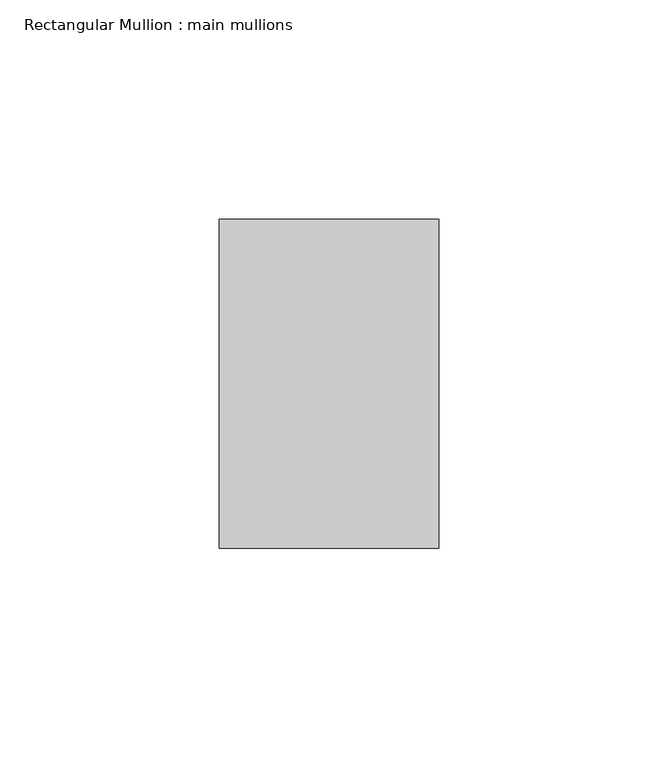
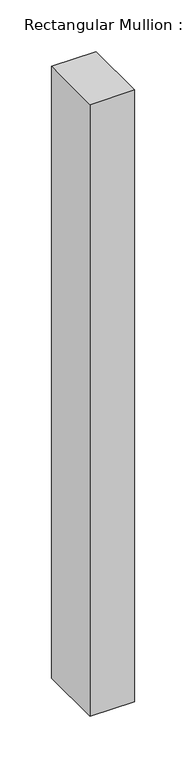
"""IFC4 building model written with IfcOpenShell, lengths in millimetres: member geometry, Rectangular Mullion : main mullions."""

from ifc_helpers import new_model, si_unit, frame, origin, place, context, project, spatial, polyline, outline, extrude, source, transform, mapped, element, save


def rectangular_mullion_main_mullions_07477f58(model_context):
    return source(origin(), model_context, "Body", "SweptSolid", [
        extrude(outline(polyline([(0.0, 37.5), (0.0, -37.5), (-50.0, -37.5), (-50.0, 37.5), (0.0, 37.5)])), frame((0.0, 0.0, -725.0), z_axis=(0.0, 0.0, 1.0), x_axis=(1.0, 0.0, 0.0)), (0.0, 0.0, 1.0), 725.0),
    ])


if __name__ == "__main__":
    model = new_model("IFC4")
    model_context = context("Model", 3, world=origin())
    ifc_project = project(units=[si_unit("LENGTHUNIT", "METRE", prefix="MILLI")], contexts=[model_context])
    site = spatial("IfcSite", under=ifc_project)
    building = spatial("IfcBuilding", under=site)
    placement = place(None, origin())
    rectangular_mullion_main_mullions_shape = rectangular_mullion_main_mullions_07477f58(model_context)
    element("IfcMember", 1, ObjectType="Rectangular Mullion : main mullions", at=placement, inside=building, context=model_context, shape_type="MappedRepresentation", body=[
        mapped(rectangular_mullion_main_mullions_shape, transform((0.0, 0.0, 0.0), x_axis=(1.0, 0.0, 0.0), y_axis=(0.0, 1.0, 0.0), z_axis=(0.0, 0.0, 1.0))),
    ])
    save(model, "model.ifc")

# Revit data of these elements
# Type "Rectangular Mullion : main mullions"
#   built-in parameter 1007304 = 0.246063 (stored number, unit not read)
#   built-in parameter 1007301 = 0.082021 (stored number, unit not read)
#   built-in parameter 1007300 = 0.082021 (stored number, unit not read)
# Element 1 (IfcMember, "Rectangular Mullion : main mullions")
#   Materials on its faces: "Aluminum"
# Materials
#   "Aluminum": class "Metal", colour RGB 136 136 136, transparency 0, Description = "Aluminum 6061", Cost = 0
